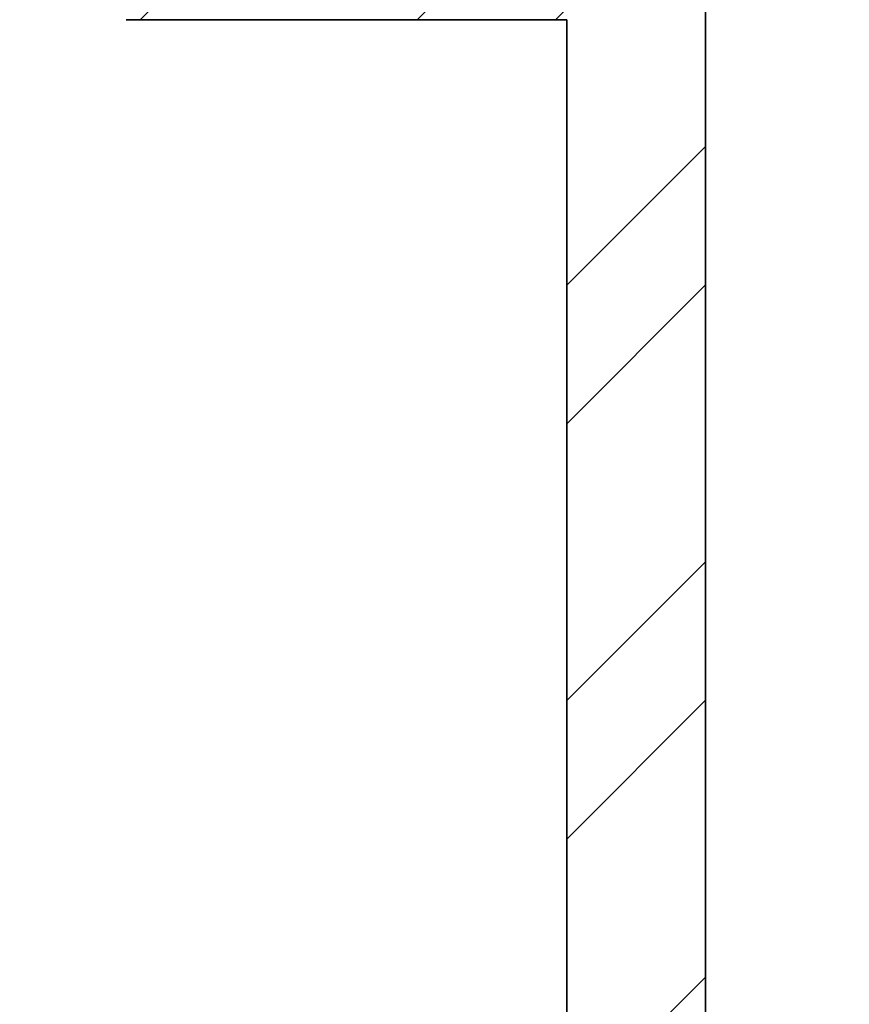
# Model space of a CAD drawing. Units: inches. Extents: x 1885 to 2748, y 783 to 2421.
# Tile 93 of 117: x 2341 to 2368, y 2282 to 2314. Entities that reach past the tile are written whole.
import ezdxf

# ---------------------------------------------------------------- set-up
doc = ezdxf.new("R2010")
doc.units = ezdxf.units.IN
doc.layers.add('A-WALL', color=7, linetype='Continuous', lineweight=35)
doc.layers.add('A-WALL-PATT', color=85, linetype='Continuous', lineweight=13, true_color=0x58ba48)

msp = doc.modelspace()

# ---------------------------------------------------------------- hatches: boundary and pattern name
at = {"layer": 'A-WALL-PATT'}
h = msp.add_hatch(dxfattribs=at)
h.set_pattern_fill('ANSI32', color=256)
h.paths.add_polyline_path([(2007.772, 2318.006), (1980.774, 2318.006), (1980.774, 2281.215), (1985.274, 2281.215), (1985.274, 2313.506), (2007.772, 2313.506), (2007.772, 2315.756)])
h.paths.add_polyline_path([(2094.324, 2318.006), (2067.772, 2318.006), (2067.772, 2313.506), (2094.324, 2313.506), (2094.324, 2315.756)])
h.paths.add_polyline_path([(2131.367, 2315.756), (2131.367, 2318.006), (2131.189, 2318.006), (2112.609, 2318.006), (2112.609, 2313.506), (2117.274, 2313.506), (2117.274, 2255.201), (2121.774, 2255.201), (2121.774, 2313.506), (2131.367, 2313.506)])
h.paths.add_polyline_path([(2190.512, 2318.006), (2155.367, 2318.006), (2155.367, 2313.506), (2169.774, 2313.506), (2169.774, 2229.506), (2121.774, 2229.506), (2121.774, 2233.451), (2119.524, 2233.451), (2117.274, 2233.451), (2117.274, 2201.101), (2121.774, 2201.101), (2121.774, 2225.006), (2169.774, 2225.006), (2169.774, 2165.006), (2306.274, 2165.006), (2306.274, 2066.006), (2310.774, 2066.006), (2344.274, 2066.006), (2486.274, 2066.006), (2486.274, 1886.006), (2483.02, 1886.006), (2483.02, 1881.506), (2486.274, 1881.506), (2486.274, 1880.678), (2490.774, 1880.678), (2490.774, 2070.506), (2344.274, 2070.506), (2310.774, 2070.506), (2310.774, 2165.006), (2310.774, 2173.636), (2308.524, 2173.636), (2306.274, 2173.636), (2306.274, 2169.506), (2174.274, 2169.506), (2174.274, 2313.506), (2190.512, 2313.506), (2190.512, 2315.756)])
h.paths.add_polyline_path([(1985.274, 2221.215), (1980.774, 2221.215), (1980.774, 2165.006), (1992.774, 2165.006), (1992.774, 2141.927), (1997.274, 2141.927), (1997.274, 2165.006), (2117.274, 2165.006), (2117.274, 2163.126), (2121.774, 2163.126), (2121.774, 2172.734), (2119.524, 2172.734), (2117.274, 2172.734), (2117.274, 2169.506), (1985.274, 2169.506)])
h.paths.add_polyline_path([(1997.274, 2105.927), (1992.774, 2105.927), (1992.774, 2070.506), (2016.774, 2070.506), (2016.774, 2059.123), (2019.024, 2059.123), (2021.274, 2059.123), (2021.274, 2070.506), (2117.274, 2070.506), (2117.274, 2022.506), (2114.423, 2022.506), (2114.423, 2018.006), (2123.627, 2018.006), (2123.627, 2020.256), (2123.627, 2022.506), (2121.774, 2022.506), (2121.774, 2142.587), (2119.524, 2142.587), (2117.274, 2142.587), (2117.274, 2075.006), (1997.274, 2075.006)])
h.paths.add_polyline_path([(2092.029, 2020.256), (2092.029, 2022.506), (2021.274, 2022.506), (2021.274, 2035.123), (2016.774, 2035.123), (2016.774, 2018.006), (2016.774, 1978.784), (2021.274, 1978.784), (2021.274, 2018.006), (2092.029, 2018.006)])
h.paths.add_polyline_path([(2260.938, 2022.506), (2153.105, 2022.506), (2153.105, 2020.256), (2153.105, 2018.006), (2155.274, 2018.006), (2155.274, 1886.006), (2107.629, 1886.006), (2107.629, 1881.506), (2182.911, 1881.506), (2182.911, 1883.756), (2182.911, 1886.006), (2159.774, 1886.006), (2159.774, 2018.006), (2260.938, 2018.006), (2260.938, 2020.256)])
h.paths.add_polyline_path([(2047.629, 1883.756), (2047.629, 1886.006), (2021.274, 1886.006), (2021.274, 1918.784), (2019.024, 1918.784), (2016.774, 1918.784), (2016.774, 1881.506), (2047.629, 1881.506)])
h.paths.add_polyline_path([(2306.361, 1883.756), (2306.361, 1886.006), (2296.274, 1886.006), (2296.274, 1982.006), (2316.535, 1982.006), (2316.535, 1984.256), (2316.535, 1986.506), (2296.274, 1986.506), (2296.274, 2022.506), (2289.276, 2022.506), (2289.276, 2018.006), (2291.774, 2018.006), (2291.774, 1886.006), (2242.911, 1886.006), (2242.911, 1881.506), (2306.361, 1881.506)], flags=17)
h.paths.add_polyline_path([(1985.274, 1843.006), (2021.6, 1843.006), (2021.534, 1845.441), (2021.477, 1847.506), (1980.774, 1847.506), (1980.774, 1809.446), (1985.274, 1809.446)])
h.paths.add_polyline_path([(2131.482, 1845.256), (2131.482, 1847.506), (2081.534, 1847.506), (2081.534, 1843.006), (2117.274, 1843.006), (2117.274, 1784.147), (2119.524, 1784.147), (2121.774, 1784.147), (2121.774, 1843.006), (2131.482, 1843.006)])
h.paths.add_polyline_path([(2203.886, 1847.506), (2155.482, 1847.506), (2155.482, 1843.006), (2169.774, 1843.006), (2169.774, 1759.006), (2121.774, 1759.006), (2121.774, 1761.457), (2117.274, 1761.457), (2117.274, 1730.429), (2121.774, 1730.429), (2121.774, 1754.506), (2177.421, 1754.506), (2177.421, 1756.756), (2177.421, 1759.006), (2174.274, 1759.006), (2174.274, 1843.006), (2203.886, 1843.006)])
h.paths.add_polyline_path([(2335.554, 1845.256), (2335.554, 1847.506), (2239.886, 1847.506), (2239.886, 1843.006), (2306.274, 1843.006), (2306.274, 1759.006), (2199.486, 1759.006), (2199.486, 1754.506), (2310.774, 1754.506), (2310.774, 1843.006), (2335.554, 1843.006)])
h.paths.add_polyline_path([(2348.774, 2022.506), (2344.274, 2022.506), (2344.274, 1986.506), (2341.681, 1986.506), (2341.681, 1982.006), (2344.274, 1982.006), (2344.274, 1886.006), (2330.361, 1886.006), (2330.361, 1881.506), (2361.627, 1881.506), (2361.627, 1883.756), (2361.627, 1886.006), (2348.774, 1886.006)], flags=17)
h.paths.add_polyline_path([(2283.251, 2315.756), (2283.251, 2318.006), (2238.512, 2318.006), (2238.512, 2313.506), (2283.251, 2313.506)], flags=17)
h.paths.add_polyline_path([(2363.274, 2348.006), (2388.677, 2348.006), (2388.677, 2350.256), (2388.677, 2352.506), (2358.774, 2352.506), (2358.774, 2348.006), (2358.774, 2318.006), (2344.481, 2318.006), (2344.481, 2313.506), (2358.774, 2313.506), (2358.774, 2229.506), (2310.774, 2229.506), (2310.774, 2231.952), (2306.274, 2231.952), (2306.274, 2205.611), (2310.774, 2205.611), (2310.774, 2225.006), (2358.774, 2225.006), (2358.774, 2211.506), (2452.329, 2211.506), (2452.329, 2213.756), (2452.329, 2216.006), (2363.274, 2216.006), (2363.274, 2318.006)])
h.paths.add_polyline_path([(2310.774, 2313.506), (2320.481, 2313.506), (2320.481, 2315.756), (2320.481, 2318.006), (2302.728, 2318.006), (2302.728, 2313.506), (2306.274, 2313.506), (2306.274, 2251.076), (2310.774, 2251.076)], flags=17)
h.paths.add_polyline_path([(2490.774, 2352.506), (2486.274, 2352.506), (2448.677, 2352.506), (2448.677, 2348.006), (2486.274, 2348.006), (2486.274, 2318.006), (2486.274, 2216.006), (2481.78, 2216.006), (2481.78, 2211.506), (2486.274, 2211.506), (2486.274, 2165.006), (2493.289, 2165.006), (2493.289, 2167.256), (2493.289, 2169.506), (2490.774, 2169.506), (2490.774, 2313.506), (2494.429, 2313.506), (2494.429, 2318.006), (2490.774, 2318.006)])
h.paths.add_polyline_path([(2534.653, 2318.006), (2515.691, 2318.006), (2515.691, 2313.506), (2534.653, 2313.506), (2534.653, 2315.756)])
h.paths.add_polyline_path([(2618.274, 2318.006), (2594.653, 2318.006), (2594.653, 2313.506), (2613.774, 2313.506), (2613.774, 2281.706), (2618.274, 2281.706)])
h.paths.add_polyline_path([(2618.274, 2221.706), (2613.774, 2221.706), (2613.774, 2169.506), (2554.019, 2169.506), (2554.019, 2165.006), (2613.774, 2165.006), (2613.774, 2152.878), (2618.274, 2152.878)])
h.paths.add_polyline_path([(2618.274, 2128.878), (2616.024, 2128.878), (2613.774, 2128.878), (2613.774, 2117.006), (2529.774, 2117.006), (2529.774, 2165.006), (2532.848, 2165.006), (2532.848, 2169.506), (2522.867, 2169.506), (2522.867, 2165.006), (2525.274, 2165.006), (2525.274, 2117.006), (2525.274, 2112.506), (2525.274, 2108.576), (2529.774, 2108.576), (2529.774, 2112.506), (2613.774, 2112.506), (2613.774, 2080.19), (2618.274, 2080.19)])
h.paths.add_polyline_path([(2618.274, 2044.19), (2616.024, 2044.19), (2613.774, 2044.19), (2613.774, 2015.506), (2529.774, 2015.506), (2529.774, 2088.582), (2527.524, 2088.582), (2525.274, 2088.582), (2525.274, 2011.006), (2613.774, 2011.006), (2613.774, 1956.755), (2618.274, 1956.755)])
h.paths.add_polyline_path([(2618.274, 1881.506), (2618.274, 1896.755), (2613.774, 1896.755), (2613.774, 1881.506), (2613.774, 1847.506), (2592.715, 1847.506), (2592.715, 1843.006), (2613.774, 1843.006), (2613.774, 1765.006), (2613.774, 1760.506), (2609.621, 1760.506), (2609.621, 1756.006), (2613.774, 1756.006), (2613.774, 1660.006), (2608.544, 1660.006), (2608.544, 1655.506), (2613.774, 1655.506), (2613.774, 1508.158), (2618.274, 1508.158)])
h.paths.add_polyline_path([(2565.774, 1843.006), (2568.997, 1843.006), (2568.997, 1847.506), (2490.774, 1847.506), (2490.774, 1849.7), (2488.524, 1849.7), (2486.274, 1849.7), (2486.274, 1847.506), (2477.274, 1847.506), (2477.274, 1838.506), (2477.274, 1821.493), (2486.274, 1821.493), (2486.274, 1838.506), (2561.274, 1838.506), (2561.274, 1765.006), (2486.274, 1765.006), (2486.274, 1786.157), (2477.274, 1786.157), (2477.274, 1765.006), (2477.274, 1756.006), (2486.274, 1756.006), (2565.774, 1756.006), (2585.621, 1756.006), (2585.621, 1758.256), (2585.621, 1760.506), (2565.774, 1760.506), (2565.774, 1765.006)])
h.paths.add_polyline_path([(2486.274, 1651.006), (2561.274, 1651.006), (2561.274, 1567.006), (2486.274, 1567.006), (2486.274, 1591.321), (2477.274, 1591.321), (2477.274, 1567.006), (2477.274, 1558.006), (2477.274, 1555.439), (2481.774, 1555.439), (2481.774, 1558.006), (2568.653, 1558.006), (2568.653, 1560.256), (2568.653, 1562.506), (2565.774, 1562.506), (2565.774, 1655.506), (2584.544, 1655.506), (2584.544, 1657.756), (2584.544, 1660.006), (2565.774, 1660.006), (2486.274, 1660.006), (2477.274, 1660.006), (2477.274, 1651.006), (2477.274, 1632.989), (2486.274, 1632.989)])
h.paths.add_polyline_path([(2449.967, 1883.756), (2449.967, 1886.006), (2421.627, 1886.006), (2421.627, 1881.506), (2449.967, 1881.506)], flags=17)
h.paths.add_polyline_path([(2447.274, 1847.506), (2395.554, 1847.506), (2395.554, 1843.006), (2442.774, 1843.006), (2442.774, 1809.27), (2447.274, 1809.27)])
h.paths.add_polyline_path([(1985.274, 1749.446), (1980.774, 1749.446), (1980.774, 1694.504), (1985.274, 1694.504), (1985.274, 1694.506), (1986.897, 1694.506), (1986.897, 1697.78), (1986.897, 1699.006), (1985.274, 1699.006)])
h.paths.add_polyline_path([(2152.774, 1699.006), (2121.774, 1699.006), (2121.774, 1703.668), (2119.524, 1703.668), (2117.274, 1703.668), (2117.274, 1699.006), (2009.219, 1699.006), (2009.219, 1694.506), (2148.274, 1694.506), (2148.274, 1692.631), (2152.774, 1692.631)])
h.paths.add_polyline_path([(2016.274, 1694.506), (2011.774, 1694.506), (2011.774, 1558.006), (2040.806, 1558.006), (2040.806, 1560.256), (2040.806, 1562.506), (2016.274, 1562.506)])
h.paths.add_polyline_path([(2152.774, 1663.017), (2150.524, 1663.017), (2148.274, 1663.017), (2148.274, 1562.506), (2100.806, 1562.506), (2100.806, 1558.006), (2165.119, 1558.006), (2165.119, 1560.256), (2165.119, 1562.506), (2152.774, 1562.506), (2152.774, 1610.506), (2224.774, 1610.506), (2224.774, 1607.99), (2229.274, 1607.99), (2229.274, 1615.006), (2152.774, 1615.006)])
h.paths.add_polyline_path([(2238.613, 1560.256), (2238.613, 1562.506), (2229.274, 1562.506), (2229.274, 1588.756), (2227.024, 1588.763), (2224.774, 1588.771), (2224.774, 1562.506), (2189.119, 1562.506), (2189.119, 1558.006), (2238.613, 1558.006)])
h.paths.add_polyline_path([(2336.024, 1560.256), (2336.024, 1562.506), (2310.774, 1562.506), (2310.774, 1656.347), (2308.524, 1656.347), (2306.274, 1656.347), (2306.274, 1562.506), (2286.613, 1562.506), (2286.613, 1558.006), (2336.024, 1558.006)])
h.paths.add_polyline_path([(2447.274, 1690.968), (2445.024, 1690.968), (2442.774, 1690.968), (2442.774, 1687.006), (2306.274, 1687.006), (2306.274, 1680.75), (2310.774, 1680.75), (2310.774, 1682.506), (2442.774, 1682.506), (2442.774, 1562.506), (2396.024, 1562.506), (2396.024, 1558.006), (2447.274, 1558.006)])
h.paths.add_polyline_path([(2447.274, 1749.27), (2445.024, 1749.27), (2442.774, 1749.27), (2442.774, 1717.232), (2447.274, 1717.232)])
h.paths.add_polyline_path([(2044.674, 1521.756), (2044.674, 1524.006), (2007.274, 1524.006), (2007.274, 1503.49), (2009.524, 1503.49), (2011.774, 1503.49), (2011.774, 1519.506), (2044.674, 1519.506)])
h.paths.add_polyline_path([(2177.969, 1521.756), (2177.969, 1524.006), (2104.674, 1524.006), (2104.674, 1519.506), (2145.774, 1519.506), (2145.774, 1387.506), (2143.37, 1387.506), (2143.37, 1383.006), (2251.585, 1383.006), (2251.585, 1385.256), (2251.585, 1387.506), (2150.274, 1387.506), (2150.274, 1519.506), (2177.969, 1519.506)])
h.paths.add_polyline_path([(2298.704, 1524.006), (2237.969, 1524.006), (2237.969, 1519.506), (2282.274, 1519.506), (2282.274, 1387.506), (2279.683, 1387.506), (2279.683, 1383.006), (2286.774, 1383.006), (2286.774, 1419.006), (2312.451, 1419.006), (2312.451, 1421.256), (2312.451, 1423.506), (2286.774, 1423.506), (2286.774, 1519.506), (2298.704, 1519.506), (2298.704, 1521.722)], flags=17)
h.paths.add_polyline_path([(2361.897, 1521.756), (2361.897, 1524.006), (2322.704, 1524.006), (2322.704, 1519.506), (2334.774, 1519.506), (2334.774, 1423.506), (2331.93, 1423.506), (2331.93, 1419.006), (2334.774, 1419.006), (2334.774, 1387.506), (2334.774, 1383.228), (2339.274, 1383.228), (2339.274, 1387.506), (2339.274, 1519.506), (2361.897, 1519.506)], flags=17)
h.paths.add_polyline_path([(2447.274, 1521.756), (2447.274, 1524.006), (2421.897, 1524.006), (2421.897, 1519.506), (2447.274, 1519.506)], flags=17)
h.paths.add_polyline_path([(2481.774, 1529.6), (2479.524, 1529.6), (2477.274, 1529.6), (2477.274, 1524.006), (2474.489, 1524.006), (2474.489, 1519.506), (2477.274, 1519.506), (2477.274, 1334.506), (2296.774, 1334.506), (2296.774, 1240.506), (2160.274, 1240.506), (2160.274, 1180.506), (2112.274, 1180.506), (2112.274, 1207.692), (2110.024, 1207.692), (2107.774, 1207.692), (2107.774, 1171.609), (2112.274, 1171.609), (2112.274, 1176.006), (2160.274, 1176.006), (2160.274, 1092.006), (2144.221, 1092.006), (2144.221, 1087.506), (2189.497, 1087.506), (2189.497, 1089.756), (2189.497, 1092.006), (2164.774, 1092.006), (2164.774, 1236.006), (2296.774, 1236.006), (2296.774, 1231.912), (2301.274, 1231.912), (2301.274, 1330.006), (2481.774, 1330.006), (2481.774, 1387.506)])
h.paths.add_polyline_path([(2618.274, 1448.158), (2613.774, 1448.158), (2613.774, 1382.506), (2529.774, 1382.506), (2525.274, 1382.506), (2525.274, 1307.062), (2529.774, 1307.062), (2529.774, 1378.006), (2613.774, 1378.006), (2613.774, 1354.988), (2618.274, 1354.988)])
h.paths.add_polyline_path([(2618.274, 1318.988), (2613.774, 1318.988), (2613.774, 1281.006), (2529.774, 1281.006), (2529.774, 1283.786), (2527.524, 1283.786), (2525.274, 1283.786), (2525.274, 1228.506), (2516.794, 1228.506), (2516.794, 1224.006), (2533.484, 1224.006), (2533.484, 1226.256), (2533.484, 1228.506), (2529.774, 1228.506), (2529.774, 1276.506), (2613.774, 1276.506), (2613.774, 1266.02), (2618.274, 1266.02)])
h.paths.add_polyline_path([(2618.274, 1134.964), (2613.774, 1134.964), (2613.774, 1092.006), (2594.545, 1092.006), (2594.545, 1087.506), (2618.274, 1087.506)])
h.paths.add_polyline_path([(2534.545, 1092.006), (2509.765, 1092.006), (2509.765, 1087.506), (2534.545, 1087.506), (2534.545, 1089.756)])
h.paths.add_polyline_path([(2481.274, 1224.006), (2484.117, 1224.006), (2484.117, 1226.256), (2484.117, 1228.506), (2476.774, 1228.506), (2476.774, 1198.506), (2471.61, 1198.506), (2471.61, 1194.006), (2476.774, 1194.006), (2476.774, 1062.006), (2436.894, 1062.006), (2436.894, 1057.506), (2476.774, 1057.506), (2481.274, 1057.506), (2481.274, 1062.006), (2481.274, 1087.506), (2485.354, 1087.506), (2485.354, 1089.756), (2485.354, 1092.006), (2481.274, 1092.006), (2481.274, 1117.506)])
h.paths.add_polyline_path([(2439.898, 1198.506), (2349.274, 1198.506), (2349.274, 1194.006), (2349.274, 1180.506), (2301.274, 1180.506), (2301.274, 1201.896), (2299.024, 1201.896), (2296.774, 1201.896), (2296.774, 1172.335), (2299.024, 1172.335), (2301.274, 1172.335), (2301.274, 1176.006), (2349.274, 1176.006), (2349.274, 1092.006), (2334.452, 1092.006), (2334.452, 1087.506), (2349.274, 1087.506), (2349.274, 1057.506), (2353.774, 1057.506), (2376.894, 1057.506), (2376.894, 1059.756), (2376.894, 1062.006), (2353.774, 1062.006), (2353.774, 1087.506), (2353.774, 1180.506), (2353.774, 1194.006), (2439.898, 1194.006), (2439.898, 1196.256)])
h.paths.add_polyline_path([(2270.596, 1089.756), (2270.596, 1092.006), (2249.497, 1092.006), (2249.497, 1087.506), (2270.596, 1087.506)], flags=17)
h.paths.add_polyline_path([(2310.452, 1092.006), (2301.274, 1092.006), (2301.274, 1153.292), (2296.774, 1153.292), (2296.774, 1092.006), (2293.786, 1092.006), (2293.786, 1087.506), (2310.452, 1087.506), (2310.452, 1089.756)], flags=17)
h.paths.add_polyline_path([(2112.274, 1150.328), (2110.024, 1150.328), (2107.774, 1150.328), (2107.774, 1092.006), (2104.465, 1092.006), (2104.465, 1087.506), (2120.221, 1087.506), (2120.221, 1089.756), (2120.221, 1092.006), (2112.274, 1092.006)])
h.paths.add_polyline_path([(2082.172, 1092.006), (2058.144, 1092.006), (2058.144, 1087.506), (2082.172, 1087.506), (2082.172, 1089.756)])
h.paths.add_polyline_path([(1975.774, 1145.638), (1971.274, 1145.638), (1971.274, 1087.506), (1980.774, 1087.506), (1998.144, 1087.506), (1998.144, 1089.756), (1998.144, 1092.006), (1985.274, 1092.006), (1975.774, 1092.006)])
h.paths.add_polyline_path([(2112.274, 1244.385), (2110.024, 1244.385), (2107.774, 1244.385), (2107.774, 1240.506), (1992.274, 1240.506), (1992.274, 1271.008), (1987.774, 1271.008), (1987.774, 1240.506), (1980.774, 1240.506), (1975.774, 1240.506), (1971.274, 1240.506), (1971.274, 1205.638), (1975.774, 1205.638), (1975.774, 1236.006), (2107.774, 1236.006), (2107.774, 1233.444), (2112.274, 1233.444), (2112.274, 1236.006)])
h.paths.add_polyline_path([(2112.274, 1383.006), (2114.783, 1383.006), (2114.783, 1385.256), (2114.783, 1387.506), (2102.476, 1387.506), (2102.476, 1383.006), (2107.774, 1383.006), (2107.774, 1335.006), (2011.774, 1335.006), (2011.774, 1349.939), (2007.274, 1349.939), (2007.274, 1335.006), (1987.774, 1335.006), (1987.774, 1330.506), (1987.774, 1307.008), (1992.274, 1307.008), (1992.274, 1330.506), (2007.274, 1330.506), (2107.774, 1330.506), (2107.774, 1264.711), (2112.274, 1264.711)])
h.paths.add_polyline_path([(2077.857, 1387.506), (2011.774, 1387.506), (2011.774, 1390.036), (2009.524, 1390.036), (2007.274, 1390.036), (2007.274, 1373.939), (2011.774, 1373.939), (2011.774, 1383.006), (2077.857, 1383.006)])
h.paths.add_polyline_path([(2011.774, 1443.49), (2007.274, 1443.49), (2007.274, 1410.248), (2011.774, 1410.248)])

# ---------------------------------------------------------------- linework, layer by layer
at = {"layer": 'A-WALL'}
for p, q in [((2363.274, 2318.006), (2363.274, 2216.006)), ((2344.481, 2313.506), (2358.774, 2313.506)), ((2358.774, 2313.506), (2358.774, 2229.506))]:
    msp.add_line(p, q, dxfattribs=at)

doc.saveas('drawing.dxf')
